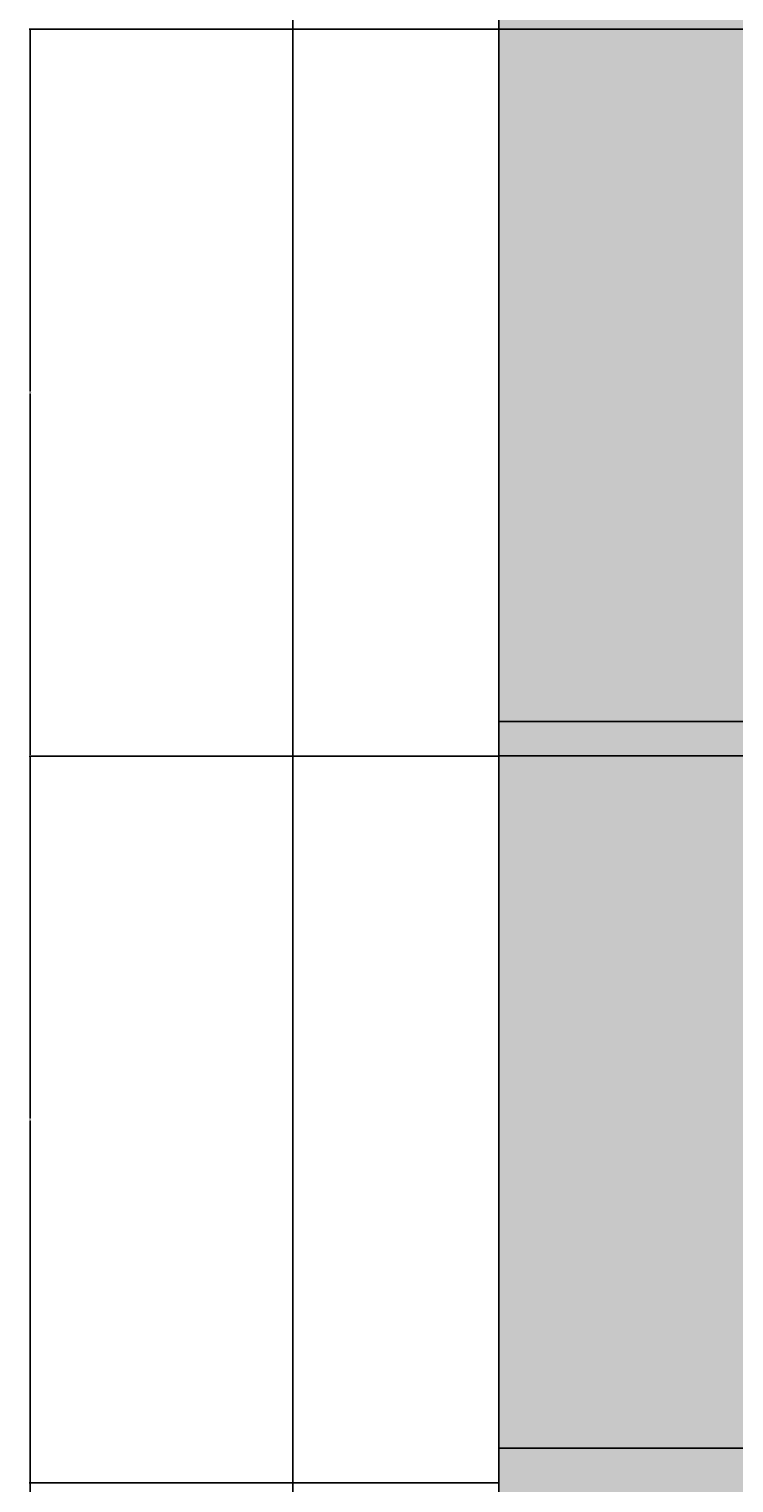
# Model space of a CAD drawing. Units: inches. Extents: x 3024 to 4744, y 1110 to 2100.
# Tile 11 of 29: x 3024 to 3146, y 1402 to 1654. Entities that reach past the tile are written whole.
import ezdxf

# ---------------------------------------------------------------- set-up
doc = ezdxf.new("R2010")
doc.units = ezdxf.units.IN
for name, color, linetype, lineweight in [('A-ANNO-DIMS', 2, 'Continuous', 18), ('A-ELEV', 7, 'Continuous', 25), ('A-ELEV-PATT', 252, 'Continuous', 13)]:
    doc.layers.add(name, color=color, linetype=linetype, lineweight=lineweight)
doc.styles.get("Standard").update_dxf_attribs({"font": 'arial.ttf'})
doc.dimstyles.get("Standard").update_dxf_attribs({"dimtxt": 0.18, "dimasz": 0.18, "dimexe": 0.18, "dimexo": 0.0625, "dimgap": 0.09, "dimtad": 0, "dimtih": 1, "dimtoh": 1, "dimdec": 1, "dimzin": 0, "dimdsep": 46, "dimlunit": 3, "dimtxsty": 'Standard', "dimcen": 0.09, "dimadec": 0, "dimazin": 0, "dimtfac": 1, "dimtdec": 1, "dimtofl": 0, "dimtmove": 0, "dimatfit": 3, "dimfxl": 1, "dimtolj": 1, "dimtzin": 0, "dimarcsym": 0})

# ---------------------------------------------------------------- blocks, each defined once
blk = doc.blocks.new('*D64')
at = {"layer": 'A-ANNO-DIMS', "color": 0, "lineweight": -2, "transparency": 16777216}
for p, q in [((3069.79, 1241.5), (3069.79, 2100.44)), ((3069.97, 2100.26), (3405.08, 2100.26)), ((3740.97, 2100.26), (3405.87, 2100.26)), ((3741.15, 1241.5), (3741.15, 2100.44))]:
    blk.add_line(p, q, dxfattribs=at)
at = {"layer": 'A-ANNO-DIMS', "color": 0, "transparency": 16777216}
for points in [[(3069.97, 2100.29), (3069.97, 2100.23), (3069.79, 2100.26)], [(3740.97, 2100.29), (3740.97, 2100.23), (3741.15, 2100.26)]]:
    blk.add_solid(points, dxfattribs=at)
at = {"layer": 'Defpoints', "color": 0, "transparency": 16777216}
for p in [(3741.15, 2100.26), (3069.79, 1241.43), (3741.15, 1241.43)]:
    blk.add_point(p, dxfattribs=at)
at = {"layer": 'A-ANNO-DIMS', "color": 0, "transparency": 16777216, "insert": (3405.47, 2100.26), "char_height": 0.18, "attachment_point": 5}
blk.add_mtext('\\A1;671.4', dxfattribs=at)
blk = doc.blocks.new('*D67')
at = {"layer": 'A-ANNO-DIMS', "color": 0, "lineweight": -2, "transparency": 16777216}
for p, q in [((3105.41, 1401.61), (3024.11, 1401.61)), ((3024.29, 1401.43), (3024.29, 1338.79)), ((3024.29, 1275.79), (3024.29, 1338.43)), ((3105.41, 1275.61), (3024.11, 1275.61))]:
    blk.add_line(p, q, dxfattribs=at)
at = {"layer": 'A-ANNO-DIMS', "color": 0, "transparency": 16777216}
for points in [[(3024.26, 1401.43), (3024.32, 1401.43), (3024.29, 1401.61)], [(3024.26, 1275.79), (3024.32, 1275.79), (3024.29, 1275.61)]]:
    blk.add_solid(points, dxfattribs=at)
at = {"layer": 'Defpoints', "color": 0, "transparency": 16777216}
for p in [(3024.29, 1401.61), (3105.47, 1401.61), (3105.47, 1275.61)]:
    blk.add_point(p, dxfattribs=at)
at = {"layer": 'A-ANNO-DIMS', "color": 0, "transparency": 16777216, "insert": (3024.29, 1338.61), "char_height": 0.18, "attachment_point": 5}
blk.add_mtext('\\A1;126', dxfattribs=at)
blk = doc.blocks.new('*D68')
at = {"layer": 'A-ANNO-DIMS', "color": 0, "lineweight": -2, "transparency": 16777216}
for p, q in [((3105.41, 1527.61), (3024.11, 1527.61)), ((3024.29, 1527.43), (3024.29, 1464.79)), ((3024.29, 1401.79), (3024.29, 1464.43)), ((3105.41, 1401.61), (3024.11, 1401.61))]:
    blk.add_line(p, q, dxfattribs=at)
at = {"layer": 'A-ANNO-DIMS', "color": 0, "transparency": 16777216}
for points in [[(3024.26, 1527.43), (3024.32, 1527.43), (3024.29, 1527.61)], [(3024.26, 1401.79), (3024.32, 1401.79), (3024.29, 1401.61)]]:
    blk.add_solid(points, dxfattribs=at)
at = {"layer": 'Defpoints', "color": 0, "transparency": 16777216}
for p in [(3024.29, 1527.61), (3105.47, 1527.61), (3105.47, 1401.61)]:
    blk.add_point(p, dxfattribs=at)
at = {"layer": 'A-ANNO-DIMS', "color": 0, "transparency": 16777216, "insert": (3024.29, 1464.61), "char_height": 0.18, "attachment_point": 5}
blk.add_mtext('\\A1;126', dxfattribs=at)
blk = doc.blocks.new('*D69')
at = {"layer": 'A-ANNO-DIMS', "color": 0, "lineweight": -2, "transparency": 16777216}
for p, q in [((3105.41, 1653.61), (3024.11, 1653.61)), ((3024.29, 1653.43), (3024.29, 1590.79)), ((3024.29, 1527.79), (3024.29, 1590.43)), ((3105.41, 1527.61), (3024.11, 1527.61))]:
    blk.add_line(p, q, dxfattribs=at)
at = {"layer": 'A-ANNO-DIMS', "color": 0, "transparency": 16777216}
for points in [[(3024.26, 1653.43), (3024.32, 1653.43), (3024.29, 1653.61)], [(3024.26, 1527.79), (3024.32, 1527.79), (3024.29, 1527.61)]]:
    blk.add_solid(points, dxfattribs=at)
at = {"layer": 'Defpoints', "color": 0, "transparency": 16777216}
for p in [(3024.29, 1653.61), (3105.47, 1653.61), (3105.47, 1527.61)]:
    blk.add_point(p, dxfattribs=at)
at = {"layer": 'A-ANNO-DIMS', "color": 0, "transparency": 16777216, "insert": (3024.29, 1590.61), "char_height": 0.18, "attachment_point": 5}
blk.add_mtext('\\A1;126', dxfattribs=at)

msp = doc.modelspace()

# ---------------------------------------------------------------- hatches: boundary and pattern name
at = {"layer": 'A-ELEV-PATT'}
h = msp.add_hatch(color=256, dxfattribs=at)
h.dxf.hatch_style = 1
h.paths.add_polyline_path([(3329.7033, 1407.6112), (3105.4722, 1407.6112), (3105.4722, 1401.6112), (3329.7033, 1401.6112)])
h.paths.add_polyline_path([(3329.7033, 1281.6112), (3105.4722, 1281.6112), (3105.4722, 1275.6112), (3112.3838, 1275.6112), (3329.7033, 1275.6112)])
h.paths.add_polyline_path([(3329.7033, 1533.6112), (3105.4722, 1533.6112), (3105.4722, 1527.6112), (3329.7033, 1527.6112)])
h.paths.add_polyline_path([(3329.7033, 1659.6112), (3105.4722, 1659.6112), (3105.4722, 1653.6112), (3329.7033, 1653.6112)])
h.paths.add_polyline_path([(3329.7033, 1785.6112), (3105.4722, 1785.6112), (3105.4722, 1779.6112), (3329.7033, 1779.6112)])
h.paths.add_polyline_path([(3329.7033, 1911.6112), (3105.4722, 1911.6112), (3095.7158, 1911.6112), (3095.7158, 1905.6112), (3329.7033, 1905.6112)])
h.paths.add_polyline_path([(3715.2286, 1911.6112), (3705.4722, 1911.6112), (3705.4722, 1905.6112), (3715.2286, 1905.6112)])
h.paths.add_polyline_path([(3688.5588, 1911.6112), (3481.2411, 1911.6112), (3481.2411, 1905.6112), (3688.5588, 1905.6112)])
h = msp.add_hatch(color=256, dxfattribs=at)
h.dxf.hatch_style = 1
h.paths.add_polyline_path([(3154.3287, 1897.4879), (3148.9694, 1897.4879), (3148.9694, 1905.6112), (3105.4722, 1905.6112), (3105.4722, 1785.6112), (3148.9694, 1785.6112), (3148.9694, 1795.0431), (3151.6604, 1795.0431), (3151.6604, 1806.8674), (3154.3287, 1806.8674)])
h.paths.add_polyline_path([(3329.7033, 1905.6112), (3292.6051, 1905.6112), (3292.6051, 1897.4879), (3287.2458, 1897.4879), (3287.2458, 1806.8674), (3288.3759, 1806.8674), (3288.3759, 1795.0431), (3292.6051, 1795.0431), (3292.6051, 1785.6112), (3329.7033, 1785.6112)])
h.paths.add_polyline_path([(3154.3287, 1771.4879), (3148.9694, 1771.4879), (3148.9694, 1779.6112), (3105.4722, 1779.6112), (3105.4722, 1659.6112), (3148.9694, 1659.6112), (3148.9694, 1669.0431), (3151.6604, 1669.0431), (3151.6604, 1680.8674), (3154.3287, 1680.8674)])
h.paths.add_polyline_path([(3329.7033, 1779.6112), (3292.6051, 1779.6112), (3292.6051, 1771.4879), (3287.2458, 1771.4879), (3287.2458, 1680.8674), (3288.3759, 1680.8674), (3288.3759, 1669.0431), (3292.6051, 1669.0431), (3292.6051, 1659.6112), (3329.7033, 1659.6112)])
h.paths.add_polyline_path([(3154.3287, 1645.4879), (3148.9694, 1645.4879), (3148.9694, 1653.6112), (3105.4722, 1653.6112), (3105.4722, 1533.6112), (3148.9694, 1533.6112), (3148.9694, 1543.0431), (3151.6604, 1543.0431), (3151.6604, 1554.8674), (3154.3287, 1554.8674)])
h.paths.add_polyline_path([(3329.7033, 1653.6112), (3292.6051, 1653.6112), (3292.6051, 1645.4879), (3287.2458, 1645.4879), (3287.2458, 1554.8674), (3288.3759, 1554.8674), (3288.3759, 1543.0431), (3292.6051, 1543.0431), (3292.6051, 1533.6112), (3329.7033, 1533.6112)])
h.paths.add_polyline_path([(3329.7033, 1527.6112), (3292.6051, 1527.6112), (3292.6051, 1519.4879), (3287.2458, 1519.4879), (3287.2458, 1428.8674), (3288.3759, 1428.8674), (3288.3759, 1417.0431), (3292.6051, 1417.0431), (3292.6051, 1407.6112), (3329.7033, 1407.6112)])
h.paths.add_polyline_path([(3329.7033, 1401.6112), (3292.6051, 1401.6112), (3292.6051, 1393.4879), (3287.2458, 1393.4879), (3287.2458, 1302.8674), (3288.3759, 1302.8674), (3288.3759, 1291.0431), (3292.6051, 1291.0431), (3292.6051, 1281.6112), (3329.7033, 1281.6112)])
h.paths.add_polyline_path([(3154.3287, 1393.4879), (3148.9694, 1393.4879), (3148.9694, 1401.6112), (3105.4722, 1401.6112), (3105.4722, 1281.6112), (3148.9694, 1281.6112), (3148.9694, 1291.0431), (3151.6604, 1291.0431), (3151.6604, 1302.8674), (3154.3287, 1302.8674)])
h.paths.add_polyline_path([(3154.3287, 1519.4879), (3148.9694, 1519.4879), (3148.9694, 1527.6112), (3105.4722, 1527.6112), (3105.4722, 1407.6112), (3148.9694, 1407.6112), (3148.9694, 1417.0431), (3151.6604, 1417.0431), (3151.6604, 1428.8674), (3154.3287, 1428.8674)])
h.paths.add_polyline_path([(3515.7606, 1897.4879), (3510.4013, 1897.4879), (3510.4013, 1905.6112), (3481.2411, 1905.6112), (3481.2411, 1785.6112), (3510.4013, 1785.6112), (3510.4013, 1795.0431), (3513.0923, 1795.0431), (3513.0923, 1806.8674), (3515.7606, 1806.8674)])
h.paths.add_polyline_path([(3688.5588, 1905.6112), (3654.037, 1905.6112), (3654.037, 1897.4879), (3648.6777, 1897.4879), (3648.6777, 1806.8674), (3649.8078, 1806.8674), (3649.8078, 1795.0431), (3654.037, 1795.0431), (3654.037, 1785.6112), (3688.5588, 1785.6112)])
h.paths.add_polyline_path([(3515.7606, 1771.4879), (3510.4013, 1771.4879), (3510.4013, 1779.6112), (3481.2411, 1779.6112), (3481.2411, 1659.6112), (3510.4013, 1659.6112), (3510.4013, 1669.0431), (3513.0923, 1669.0431), (3513.0923, 1680.8674), (3515.7606, 1680.8674)])
h.paths.add_polyline_path([(3688.5588, 1779.6112), (3654.037, 1779.6112), (3654.037, 1771.4879), (3648.6777, 1771.4879), (3648.6777, 1680.8674), (3649.8078, 1680.8674), (3649.8078, 1669.0431), (3654.037, 1669.0431), (3654.037, 1659.6112), (3688.5588, 1659.6112)])
h.paths.add_polyline_path([(3515.7606, 1645.4879), (3510.4013, 1645.4879), (3510.4013, 1653.6112), (3481.2411, 1653.6112), (3481.2411, 1533.6112), (3510.4013, 1533.6112), (3510.4013, 1543.0431), (3513.0923, 1543.0431), (3513.0923, 1554.8674), (3515.7606, 1554.8674)])
h.paths.add_polyline_path([(3688.5588, 1653.6112), (3654.037, 1653.6112), (3654.037, 1645.4879), (3648.6777, 1645.4879), (3648.6777, 1554.8674), (3649.8078, 1554.8674), (3649.8078, 1543.0431), (3654.037, 1543.0431), (3654.037, 1533.6112), (3688.5588, 1533.6112)])
h.paths.add_polyline_path([(3515.7606, 1519.4879), (3510.4013, 1519.4879), (3510.4013, 1527.6112), (3481.2411, 1527.6112), (3481.2411, 1407.6112), (3510.4013, 1407.6112), (3510.4013, 1417.0431), (3513.0923, 1417.0431), (3513.0923, 1428.8674), (3515.7606, 1428.8674)])
h.paths.add_polyline_path([(3688.5588, 1527.6112), (3654.037, 1527.6112), (3654.037, 1519.4879), (3648.6777, 1519.4879), (3648.6777, 1428.8674), (3649.8078, 1428.8674), (3649.8078, 1417.0431), (3654.037, 1417.0431), (3654.037, 1407.6112), (3688.5588, 1407.6112)])
h.paths.add_polyline_path([(3515.7606, 1393.4879), (3510.4013, 1393.4879), (3510.4013, 1401.6112), (3481.2411, 1401.6112), (3481.2411, 1281.6112), (3510.4013, 1281.6112), (3510.4013, 1291.0431), (3513.0923, 1291.0431), (3513.0923, 1302.8674), (3515.7606, 1302.8674)])
h.paths.add_polyline_path([(3688.5588, 1401.6112), (3654.037, 1401.6112), (3654.037, 1393.4879), (3648.6777, 1393.4879), (3648.6777, 1302.8674), (3649.8078, 1302.8674), (3649.8078, 1291.0431), (3654.037, 1291.0431), (3654.037, 1281.6112), (3688.5588, 1281.6112)])
h.paths.add_polyline_path([(3515.7606, 1267.4879), (3510.4013, 1267.4879), (3510.4013, 1275.6112), (3481.2411, 1275.6112), (3481.2411, 1155.6112), (3510.4013, 1155.6112), (3510.4013, 1165.0431), (3513.0923, 1165.0431), (3513.0923, 1176.8674), (3515.7606, 1176.8674)])
h.paths.add_polyline_path([(3688.5588, 1275.6112), (3654.037, 1275.6112), (3654.037, 1267.4879), (3648.6777, 1267.4879), (3648.6777, 1176.8674), (3649.8078, 1176.8674), (3649.8078, 1165.0431), (3654.037, 1165.0431), (3654.037, 1155.6112), (3688.5588, 1155.6112)])
h.paths.add_polyline_path([(3112.3838, 1275.6112), (3105.4722, 1275.6112), (3105.4722, 1171.0239), (3112.3838, 1171.0239)])

# ---------------------------------------------------------------- linework, layer by layer
at = {"layer": 'A-ELEV'}
for p, q in [((3105.4722, 1171.0239), (3105.4722, 1905.6112)), ((3105.4722, 1171.0239), (3105.4722, 1905.6112)), ((3329.7033, 1653.6112), (3105.4722, 1653.6112)), ((3329.7033, 1653.6112), (3105.4722, 1653.6112)), ((3105.4722, 1533.6112), (3329.7033, 1533.6112)), ((3105.4722, 1533.6112), (3329.7033, 1533.6112)), ((3329.7033, 1527.6112), (3105.4722, 1527.6112)), ((3329.7033, 1527.6112), (3105.4722, 1527.6112)), ((3105.4722, 1407.6112), (3329.7033, 1407.6112)), ((3105.4722, 1407.6112), (3329.7033, 1407.6112))]:
    msp.add_line(p, q, dxfattribs=at)

# ---------------------------------------------------------------- dimensions: what is measured, and where the dimension line sits
at = {"layer": 'A-ANNO-DIMS'}
dim = msp.add_linear_dim(base=(3741.1507, 2100.2584), p1=(3069.7937, 1241.4341), p2=(3741.1507, 1241.4341), dimstyle='Standard', override={"dimdec": 1, "dimlfac": 1, "dimrnd": 0, "dimzin": 0, "dimdsep": 46, "dimlunit": 2}, dxfattribs=at)
dim.commit()
dim.dimension.update_dxf_attribs({"geometry": '*D64', "text_midpoint": (3405.4722, 2100.2584)})
for base, p1, p2, picture, middle in [((3024.2937, 1653.6112), (3105.4722, 1527.6112), (3105.4722, 1653.6112), '*D69', (3024.2937, 1590.6112)), ((3024.2937, 1527.6112), (3105.4722, 1401.6112), (3105.4722, 1527.6112), '*D68', (3024.2937, 1464.6112)), ((3024.2937, 1401.6112), (3105.4722, 1275.6112), (3105.4722, 1401.6112), '*D67', (3024.2937, 1338.6112))]:
    dim = msp.add_linear_dim(base=base, p1=p1, p2=p2, angle=90, dimstyle='Standard', override={"dimdec": 0, "dimlfac": 1, "dimrnd": 0, "dimzin": 0, "dimdsep": 46, "dimlunit": 2}, dxfattribs=at)
    dim.commit()
    dim.dimension.update_dxf_attribs({"geometry": picture, "text_midpoint": middle})

doc.saveas('drawing.dxf')
